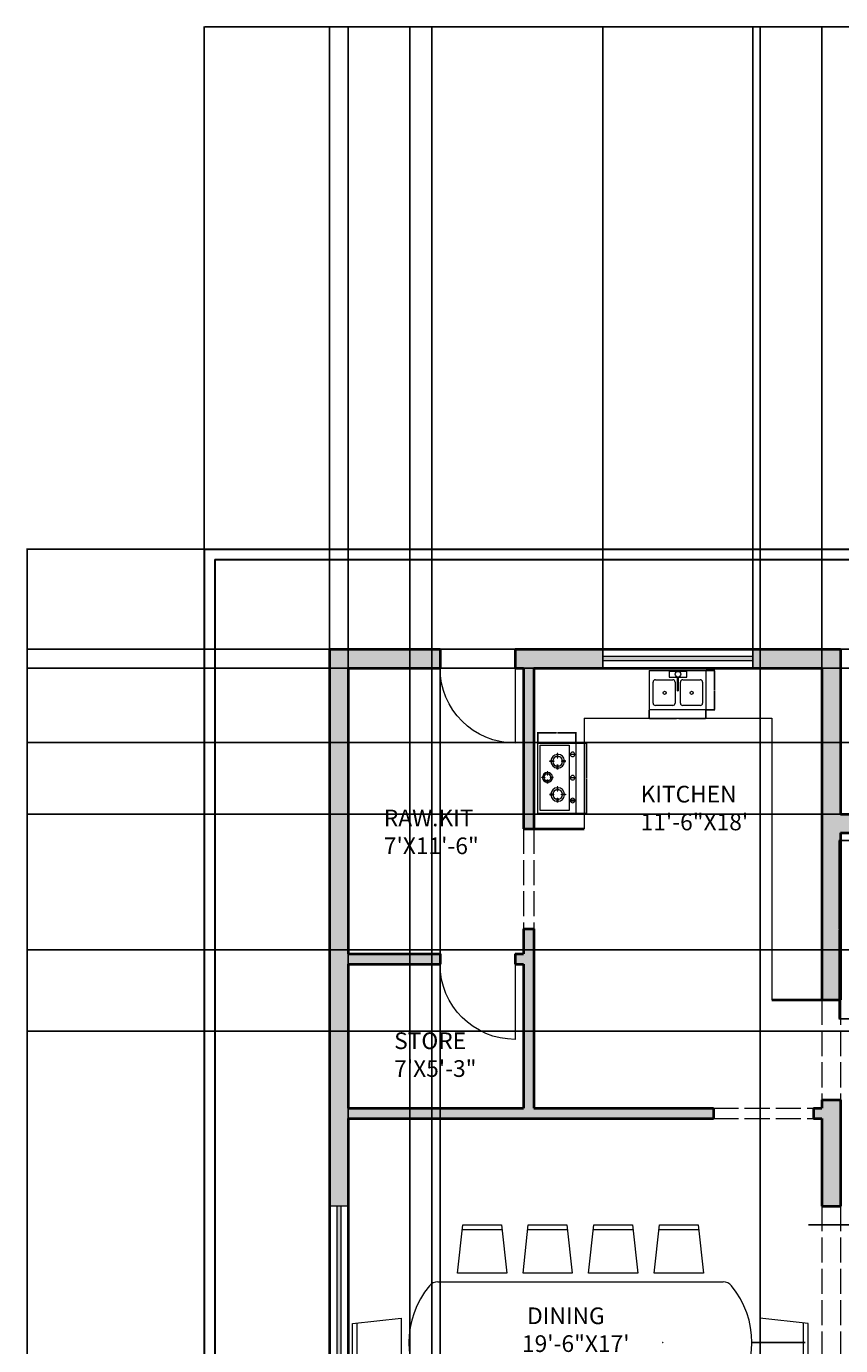
# Model space of a CAD drawing. Units: inches. Extents: x 2330 to 3943, y 1763 to 3461.
# Tile 24 of 40: x 2330 to 2721, y 2829 to 3461. Entities that reach past the tile are written whole.
import ezdxf

# ---------------------------------------------------------------- set-up
doc = ezdxf.new("R2010")
doc.units = ezdxf.units.IN
doc.linetypes.add('ACAD_ISO02W100', pattern=[15, 12, -3])
for name, color, linetype, lineweight in [('A-ANNO-DIMS', 2, 'Continuous', 18), ('A-AREA-IDEN', 7, 'Continuous', 18), ('A-DOOR', 4, 'Continuous', 18), ('A-EQPM', 9, 'Continuous', 18), ('A-FLOR-CASE', 8, 'Continuous', 18), ('A-FLOR-FIXT', 8, 'Continuous', 18), ('A-FURN', 8, 'Continuous', 13), ('A-GLAZ', 4, 'Continuous', 18), ('A-WALL', 7, 'Continuous', 40), ('A-WALL-OVHD', 7, 'ACAD_ISO02W100', 18), ('A-WALL-PATT', 252, 'Continuous', 13), ('C-PROP', 7, 'Continuous', 30)]:
    doc.layers.add(name, color=color, linetype=linetype, lineweight=lineweight)
doc.styles.get("Standard").update_dxf_attribs({"font": 'arial.ttf'})
doc.dimstyles.get("Standard").update_dxf_attribs({"dimtxt": 0.18, "dimasz": 0.18, "dimexe": 0.18, "dimexo": 0.0625, "dimgap": 0.09, "dimtad": 0, "dimtih": 1, "dimtoh": 1, "dimdec": 4, "dimzin": 0, "dimdsep": 46, "dimtxsty": 'Standard', "dimcen": 0.09, "dimadec": 0, "dimazin": 0, "dimtfac": 1, "dimtdec": 4, "dimtofl": 0, "dimtmove": 0, "dimatfit": 3, "dimfxl": 1, "dimtolj": 1, "dimtzin": 0, "dimarcsym": 0})

# ---------------------------------------------------------------- blocks, each defined once
blk = doc.blocks.new('A$C113D154D')
for p, q in [((0.96, 1.712), (1.008, 2.155)), ((1.003, 2.112), (1.367, 2.112)), ((1.008, 2.155), (1.362, 2.155)), ((1.362, 2.155), (1.41, 1.712)), ((1.56, 1.712), (1.608, 2.155)), ((1.603, 2.112), (1.967, 2.112)), ((1.608, 2.155), (1.962, 2.155)), ((1.962, 2.155), (2.01, 1.712)), ((2.16, 1.712), (2.208, 2.155)), ((2.203, 2.112), (2.567, 2.112)), ((2.208, 2.155), (2.562, 2.155)), ((2.562, 2.155), (2.61, 1.712)), ((2.76, 1.712), (2.808, 2.155)), ((2.803, 2.112), (3.167, 2.112)), ((2.808, 2.155), (3.162, 2.155)), ((3.162, 2.155), (3.21, 1.712)), ((1.41, 1.712), (0.96, 1.712)), ((2.01, 1.712), (1.56, 1.712)), ((2.61, 1.712), (2.16, 1.712)), ((3.21, 1.712), (2.76, 1.712)), ((0.78, 1.633), (3.39, 1.633)), ((0, 1.252), (0.443, 1.3)), ((0, 0.897), (0, 1.252)), ((0.043, 0.893), (0.043, 1.257)), ((0.443, 1.3), (0.443, 0.85)), ((3.727, 1.3), (3.727, 0.85)), ((4.17, 1.252), (3.727, 1.3)), ((4.127, 0.893), (4.127, 1.257)), ((4.17, 0.897), (4.17, 1.252)), ((0.443, 0.85), (0, 0.897)), ((3.727, 0.85), (4.17, 0.897)), ((3.39, 0.521), (0.78, 0.521)), ((1.41, 0.443), (0.96, 0.443)), ((0.96, 0.443), (1.008, 0)), ((1.362, 0), (1.41, 0.443)), ((2.01, 0.443), (1.56, 0.443)), ((1.56, 0.443), (1.608, 0)), ((1.962, 0), (2.01, 0.443)), ((2.61, 0.443), (2.16, 0.443)), ((2.16, 0.443), (2.208, 0)), ((2.562, 0), (2.61, 0.443)), ((3.21, 0.443), (2.76, 0.443)), ((2.76, 0.443), (2.808, 0)), ((3.162, 0), (3.21, 0.443)), ((1.003, 0.043), (1.367, 0.043)), ((1.008, 0), (1.362, 0)), ((1.603, 0.043), (1.967, 0.043)), ((1.608, 0), (1.962, 0)), ((2.203, 0.043), (2.567, 0.043)), ((2.208, 0), (2.562, 0)), ((2.803, 0.043), (3.167, 0.043)), ((2.808, 0), (3.162, 0))]:
    blk.add_line(p, q)
for centre, radius, start, end in [((1.331, 1.077), 0.815, 140.3976, 219.6024), ((0.78, 1.533), 0.1, 90, 140.3976), ((3.39, 1.533), 0.1, 39.6024, 90), ((2.839, 1.077), 0.815, 320.3976, 39.6024), ((0.78, 0.621), 0.1, 219.6024, 270), ((3.39, 0.621), 0.1, 270, 320.3976)]:
    blk.add_arc(centre, radius, start, end)
blk = doc.blocks.new('A$C72243D80')
at = {"ltscale": 1000}
for p, q in [((0, 0), (0, 384)), ((0, 384), (712, 384)), ((30, 69), (30, 363)), ((30, 363), (693, 363)), ((309, 291), (340, 291)), ((309, 285), (309, 291)), ((340, 285), (309, 285)), ((340, 291), (340, 285)), ((364, 315), (364, 345)), ((364, 345), (370, 345)), ((370, 315), (364, 315)), ((370, 345), (370, 315)), ((392, 291), (392, 285)), ((423, 291), (392, 291)), ((392, 285), (423, 285)), ((423, 285), (423, 291)), ((693, 363), (693, 69)), ((712, 384), (712, 0)), ((115, 190), (157, 190)), ((115, 182), (115, 190)), ((157, 182), (115, 182)), ((157, 190), (157, 182)), ((188, 264), (188, 222)), ((196, 264), (188, 264)), ((188, 222), (196, 222)), ((188, 147), (196, 147)), ((188, 105), (188, 147)), ((196, 222), (196, 264)), ((196, 147), (196, 105)), ((229, 190), (229, 182)), ((271, 190), (229, 190)), ((229, 182), (271, 182)), ((271, 182), (271, 190)), ((364, 260), (364, 229)), ((370, 260), (364, 260)), ((364, 229), (370, 229)), ((370, 229), (370, 260)), ((451, 190), (494, 190)), ((451, 182), (451, 190)), ((494, 182), (451, 182)), ((494, 190), (494, 182)), ((526, 222), (526, 264)), ((526, 264), (534, 264)), ((534, 222), (526, 222)), ((526, 147), (526, 105)), ((534, 147), (526, 147)), ((534, 264), (534, 222)), ((534, 105), (534, 147)), ((565, 190), (565, 182)), ((608, 190), (565, 190)), ((565, 182), (608, 182)), ((608, 182), (608, 190)), ((712, 0), (0, 0)), ((693, 69), (30, 69)), ((130, 61), (130, 5)), ((134, 61), (130, 61)), ((130, 5), (134, 5)), ((134, 5), (134, 61)), ((196, 105), (188, 105)), ((361, 5), (361, 61)), ((361, 61), (366, 61)), ((366, 5), (361, 5)), ((366, 61), (366, 5)), ((526, 105), (534, 105)), ((597, 5), (597, 61)), ((597, 61), (602, 61)), ((602, 5), (597, 5)), ((602, 61), (602, 5))]:
    blk.add_line(p, q, dxfattribs=at)
for centre, radius, start, end in [((366, 287), 50.3, 93.0344, 175.7271), ((366, 287), 50.3, 182.5783, 266.9656), ((366, 288), 36.3, 94.0374, 175.0142), ((366, 288), 36.3, 184.5153, 265.9626), ((366, 287), 50.3, 4.2729, 86.1838), ((366, 288), 36.3, 4.9858, 84.5356), ((366, 288), 36.3, 275.4644, 355.4847), ((366, 287), 50.3, 273.8162, 357.4217), ((193, 185), 69.2, 93.8162, 175.7271), ((193, 185), 69.2, 182.5783, 266.1838), ((193, 185), 49.9, 95.4644, 175.0142), ((193, 185), 49.9, 184.5153, 264.5356), ((193, 185), 69.2, 4.2729, 86.9656), ((193, 185), 49.9, 4.9858, 85.9626), ((193, 185), 49.9, 274.0374, 355.4847), ((193, 185), 69.2, 273.0344, 357.4217), ((530, 185), 69.2, 182.5783, 266.9656), ((530, 185), 69.2, 93.0344, 175.7271), ((529, 185), 49.9, 94.0374, 175.0142), ((529, 185), 49.9, 184.5153, 265.9626), ((530, 185), 69.2, 4.2729, 86.1838), ((529, 185), 49.9, 4.9858, 84.5356), ((530, 185), 69.2, 273.8162, 357.4217), ((529, 185), 49.9, 275.4644, 355.4847), ((132, 33), 22.5, 96.7453, 263.2547), ((132, 33), 22.5, 275.4789, 84.5211), ((363, 33), 22.5, 95.4789, 264.5211), ((363, 33), 22.5, 276.7453, 83.2547), ((599, 33), 22.5, 95.4789, 264.5211), ((599, 33), 22.5, 276.7453, 83.2547)]:
    blk.add_arc(centre, radius, start, end, dxfattribs=at)
blk = doc.blocks.new('A$C3AD04490')
for p, q in [((0, 641), (0, 0)), ((0, 641), (925, 641)), ((62, 111), (62, 451)), ((101, 490), (383, 490)), ((614, 627), (323, 627)), ((323, 627), (323, 532)), ((323, 532), (614, 532)), ((422, 451), (422, 111)), ((463, 312), (463, 537)), ((474, 537), (474, 312)), ((509, 111), (509, 451)), ((548, 490), (830, 490)), ((614, 532), (614, 627)), ((869, 451), (869, 111)), ((925, 641), (925, 0)), ((463, 311), (474, 311)), ((383, 72), (101, 72)), ((830, 72), (548, 72)), ((925, 0), (0, 0))]:
    blk.add_line(p, q)
for centre, radius in [((469, 581), 45.9), ((251, 278), 26.4), ((691, 278), 26.4)]:
    blk.add_circle(centre, radius)
for centre, start, end in [((101, 451), 90, 180), ((383, 451), 0, 90), ((548, 451), 90, 180), ((830, 451), 0, 90), ((101, 111), 180, 270), ((383, 111), 270, 0), ((548, 111), 180, 270), ((830, 111), 270, 0)]:
    blk.add_arc(centre, 39.1, start, end)
blk = doc.blocks.new('DOOR-SINGLE-36IN')
blk.add_line((0, 0), (-36, 0))
blk.add_arc((0, 0), 36, 180, 270)
blk = doc.blocks.new('WINDOW-120IN')
h = blk.add_hatch(color=256)
h.dxf.hatch_style = 1
h.paths.add_polyline_path([(120, 5.5), (0, 5.5), (0, 3.5), (120, 3.5)])
for p, q in [((0, 9), (0, 0)), ((120, 9), (120, 0)), ((120, 5.5), (0, 5.5)), ((120, 3.5), (0, 3.5))]:
    blk.add_line(p, q)
blk = doc.blocks.new('*D42')
at = {"layer": 'A-ANNO-DIMS', "color": 0, "lineweight": -2, "transparency": 16777216}
for p, q in [((2732.75, 3071.05), (2719.8, 3071.05)), ((2719.98, 3070.87), (2719.98, 3028.47)), ((2719.98, 2985.7), (2719.98, 3028.1)), ((2732.75, 2985.52), (2719.8, 2985.52))]:
    blk.add_line(p, q, dxfattribs=at)
at = {"layer": 'A-ANNO-DIMS', "color": 0, "transparency": 16777216}
for points in [[(2719.95, 3070.87), (2720.01, 3070.87), (2719.98, 3071.05)], [(2719.95, 2985.7), (2720.01, 2985.7), (2719.98, 2985.52)]]:
    blk.add_solid(points, dxfattribs=at)
at = {"layer": 'Defpoints', "color": 0, "transparency": 16777216}
for p in [(2719.98, 3071.05), (2732.81, 3071.05), (2732.81, 2985.52)]:
    blk.add_point(p, dxfattribs=at)
at = {"layer": 'A-ANNO-DIMS', "color": 0, "transparency": 16777216, "insert": (2719.98, 3028.29), "char_height": 0.18, "attachment_point": 5}
blk.add_mtext('\\A1;86 TYP.', dxfattribs=at)
blk = doc.blocks.new('*D52')
at = {"layer": 'A-ANNO-DIMS', "color": 0, "lineweight": -2, "transparency": 16777216}
for p, q in [((2705.22, 2886.72), (2738.1, 2886.72)), ((2737.92, 2886.54), (2737.92, 2830.48)), ((2737.92, 2774.05), (2737.92, 2830.11)), ((2705.22, 2773.87), (2738.1, 2773.87))]:
    blk.add_line(p, q, dxfattribs=at)
at = {"layer": 'A-ANNO-DIMS', "color": 0, "transparency": 16777216}
for points in [[(2737.89, 2886.54), (2737.95, 2886.54), (2737.92, 2886.72)], [(2737.89, 2774.05), (2737.95, 2774.05), (2737.92, 2773.87)]]:
    blk.add_solid(points, dxfattribs=at)
at = {"layer": 'Defpoints', "color": 0, "transparency": 16777216}
for p in [(2705.15, 2886.72), (2737.92, 2886.72), (2705.15, 2773.87)]:
    blk.add_point(p, dxfattribs=at)
at = {"layer": 'A-ANNO-DIMS', "color": 0, "transparency": 16777216, "insert": (2737.92, 2830.3), "char_height": 0.18, "attachment_point": 5}
blk.add_mtext('\\A1;113', dxfattribs=at)
blk = doc.blocks.new('*D53')
at = {"layer": 'A-ANNO-DIMS', "color": 0, "lineweight": -2, "transparency": 16777216}
for p, q in [((2593.83, 3117.63), (2599, 3117.63)), ((2598.82, 3117.45), (2598.82, 3100.96)), ((2598.82, 3084.1), (2598.82, 3100.59)), ((2593.83, 3083.92), (2599, 3083.92))]:
    blk.add_line(p, q, dxfattribs=at)
at = {"layer": 'A-ANNO-DIMS', "color": 0, "transparency": 16777216}
for points in [[(2598.79, 3117.45), (2598.85, 3117.45), (2598.82, 3117.63)], [(2598.79, 3084.1), (2598.85, 3084.1), (2598.82, 3083.92)]]:
    blk.add_solid(points, dxfattribs=at)
at = {"layer": 'Defpoints', "color": 0, "transparency": 16777216}
for p in [(2593.76, 3117.63), (2598.82, 3117.63), (2593.76, 3083.92)]:
    blk.add_point(p, dxfattribs=at)
at = {"layer": 'A-ANNO-DIMS', "color": 0, "transparency": 16777216, "insert": (2598.82, 3100.77), "char_height": 0.18, "attachment_point": 5}
blk.add_mtext('\\A1;HOB 34', dxfattribs=at)
blk = doc.blocks.new('*D54')
at = {"layer": 'A-ANNO-DIMS', "color": 0, "lineweight": -2, "transparency": 16777216}
for p, q in [((2575.57, 3117.69), (2575.57, 3122.87)), ((2575.75, 3122.69), (2584.46, 3122.69)), ((2593.58, 3122.69), (2584.88, 3122.69)), ((2593.76, 3117.69), (2593.76, 3122.87))]:
    blk.add_line(p, q, dxfattribs=at)
at = {"layer": 'A-ANNO-DIMS', "color": 0, "transparency": 16777216}
for points in [[(2575.75, 3122.72), (2575.75, 3122.66), (2575.57, 3122.69)], [(2593.58, 3122.72), (2593.58, 3122.66), (2593.76, 3122.69)]]:
    blk.add_solid(points, dxfattribs=at)
at = {"layer": 'Defpoints', "color": 0, "transparency": 16777216}
for p in [(2575.57, 3122.69), (2575.57, 3117.63), (2593.76, 3117.63)]:
    blk.add_point(p, dxfattribs=at)
at = {"layer": 'A-ANNO-DIMS', "color": 0, "transparency": 16777216, "insert": (2584.67, 3122.69), "char_height": 0.18, "attachment_point": 5}
blk.add_mtext('\\A1;18', dxfattribs=at)
blk = doc.blocks.new('*D55')
at = {"layer": 'A-ANNO-DIMS', "color": 0, "lineweight": -2, "transparency": 16777216}
for p, q in [((2628.92, 3133.56), (2628.92, 3129.36)), ((2656.13, 3133.56), (2656.13, 3129.36)), ((2629.1, 3129.54), (2641.98, 3129.54)), ((2655.95, 3129.54), (2643.07, 3129.54))]:
    blk.add_line(p, q, dxfattribs=at)
at = {"layer": 'A-ANNO-DIMS', "color": 0, "transparency": 16777216}
for points in [[(2629.1, 3129.57), (2629.1, 3129.51), (2628.92, 3129.54)], [(2655.95, 3129.57), (2655.95, 3129.51), (2656.13, 3129.54)]]:
    blk.add_solid(points, dxfattribs=at)
at = {"layer": 'Defpoints', "color": 0, "transparency": 16777216}
for p in [(2628.92, 3133.62), (2656.13, 3133.62), (2656.13, 3129.54)]:
    blk.add_point(p, dxfattribs=at)
at = {"layer": 'A-ANNO-DIMS', "color": 0, "transparency": 16777216, "insert": (2642.52, 3129.54), "char_height": 0.18, "attachment_point": 5}
blk.add_mtext('\\A1;SINK 27', dxfattribs=at)
blk = doc.blocks.new('*D56')
at = {"layer": 'A-ANNO-DIMS', "color": 0, "lineweight": -2, "transparency": 16777216}
for p, q in [((2656.19, 3152.47), (2660.39, 3152.47)), ((2660.21, 3152.29), (2660.21, 3143.23)), ((2660.21, 3133.8), (2660.21, 3142.87)), ((2656.19, 3133.62), (2660.39, 3133.62))]:
    blk.add_line(p, q, dxfattribs=at)
at = {"layer": 'A-ANNO-DIMS', "color": 0, "transparency": 16777216}
for points in [[(2660.18, 3152.29), (2660.24, 3152.29), (2660.21, 3152.47)], [(2660.18, 3133.8), (2660.24, 3133.8), (2660.21, 3133.62)]]:
    blk.add_solid(points, dxfattribs=at)
at = {"layer": 'Defpoints', "color": 0, "transparency": 16777216}
for p in [(2656.13, 3152.47), (2660.21, 3152.47), (2656.13, 3133.62)]:
    blk.add_point(p, dxfattribs=at)
at = {"layer": 'A-ANNO-DIMS', "color": 0, "transparency": 16777216, "insert": (2660.21, 3143.05), "char_height": 0.18, "attachment_point": 5}
blk.add_mtext('\\A1;19', dxfattribs=at)
blk = doc.blocks.new('*D59')
at = {"layer": 'A-ANNO-DIMS', "color": 0, "lineweight": -2, "transparency": 16777216}
for p, q in [((2415.66, 3210.71), (2415.66, 3461.3)), ((2415.84, 3461.12), (3111.31, 3461.12)), ((3807.48, 3461.12), (3112.01, 3461.12)), ((3807.66, 3210.71), (3807.66, 3461.3))]:
    blk.add_line(p, q, dxfattribs=at)
at = {"layer": 'A-ANNO-DIMS', "color": 0, "transparency": 16777216}
for points in [[(2415.84, 3461.15), (2415.84, 3461.09), (2415.66, 3461.12)], [(3807.48, 3461.15), (3807.48, 3461.09), (3807.66, 3461.12)]]:
    blk.add_solid(points, dxfattribs=at)
at = {"layer": 'Defpoints', "color": 0, "transparency": 16777216}
for p in [(3807.66, 3461.12), (2415.66, 3210.65), (3807.66, 3210.65)]:
    blk.add_point(p, dxfattribs=at)
at = {"layer": 'A-ANNO-DIMS', "color": 0, "transparency": 16777216, "insert": (3111.66, 3461.12), "char_height": 0.18, "attachment_point": 5}
blk.add_mtext('\\A1;1392', dxfattribs=at)
blk = doc.blocks.new('*D60')
at = {"layer": 'A-ANNO-DIMS', "color": 0, "lineweight": -2, "transparency": 16777216}
for p, q in [((2415.6, 3210.65), (2330.5, 3210.65)), ((2330.68, 3210.47), (2330.68, 2592.83)), ((2330.68, 1974.83), (2330.68, 2592.47)), ((2415.6, 1974.65), (2330.5, 1974.65))]:
    blk.add_line(p, q, dxfattribs=at)
at = {"layer": 'A-ANNO-DIMS', "color": 0, "transparency": 16777216}
for points in [[(2330.65, 3210.47), (2330.71, 3210.47), (2330.68, 3210.65)], [(2330.65, 1974.83), (2330.71, 1974.83), (2330.68, 1974.65)]]:
    blk.add_solid(points, dxfattribs=at)
at = {"layer": 'Defpoints', "color": 0, "transparency": 16777216}
for p in [(2330.68, 3210.65), (2415.66, 3210.65), (2415.66, 1974.65)]:
    blk.add_point(p, dxfattribs=at)
at = {"layer": 'A-ANNO-DIMS', "color": 0, "transparency": 16777216, "insert": (2330.68, 2592.65), "char_height": 0.18, "attachment_point": 5}
blk.add_mtext('\\A1;1236', dxfattribs=at)
blk = doc.blocks.new('*D61')
at = {"layer": 'A-ANNO-DIMS', "color": 0, "lineweight": -2, "transparency": 16777216}
for p, q in [((2475.66, 3162.71), (2475.66, 3461.3)), ((2475.84, 3461.12), (2965.37, 3461.12)), ((3455.48, 3461.12), (2965.95, 3461.12)), ((3455.66, 3162.71), (3455.66, 3461.3))]:
    blk.add_line(p, q, dxfattribs=at)
at = {"layer": 'A-ANNO-DIMS', "color": 0, "transparency": 16777216}
for points in [[(2475.84, 3461.15), (2475.84, 3461.09), (2475.66, 3461.12)], [(3455.48, 3461.15), (3455.48, 3461.09), (3455.66, 3461.12)]]:
    blk.add_solid(points, dxfattribs=at)
at = {"layer": 'Defpoints', "color": 0, "transparency": 16777216}
for p in [(3455.66, 3461.12), (2475.66, 3162.65), (3455.66, 3162.65)]:
    blk.add_point(p, dxfattribs=at)
at = {"layer": 'A-ANNO-DIMS', "color": 0, "transparency": 16777216, "insert": (2965.66, 3461.12), "char_height": 0.18, "attachment_point": 5}
blk.add_mtext('\\A1;980', dxfattribs=at)
blk = doc.blocks.new('*D62')
at = {"layer": 'A-ANNO-DIMS', "color": 0, "lineweight": -2, "transparency": 16777216}
for p, q in [((2475.6, 3162.65), (2330.5, 3162.65)), ((2330.68, 3162.47), (2330.68, 2687.58)), ((2330.68, 2212.33), (2330.68, 2687.22)), ((2475.6, 2212.15), (2330.5, 2212.15))]:
    blk.add_line(p, q, dxfattribs=at)
at = {"layer": 'A-ANNO-DIMS', "color": 0, "transparency": 16777216}
for points in [[(2330.65, 3162.47), (2330.71, 3162.47), (2330.68, 3162.65)], [(2330.65, 2212.33), (2330.71, 2212.33), (2330.68, 2212.15)]]:
    blk.add_solid(points, dxfattribs=at)
at = {"layer": 'Defpoints', "color": 0, "transparency": 16777216}
for p in [(2330.68, 3162.65), (2475.66, 3162.65), (2475.66, 2212.15)]:
    blk.add_point(p, dxfattribs=at)
at = {"layer": 'A-ANNO-DIMS', "color": 0, "transparency": 16777216, "insert": (2330.68, 2687.4), "char_height": 0.18, "attachment_point": 5}
blk.add_mtext('\\A1;950.5', dxfattribs=at)
blk = doc.blocks.new('*D63')
at = {"layer": 'A-ANNO-DIMS', "color": 0, "lineweight": -2, "transparency": 16777216}
for p, q in [((2415.66, 3210.71), (2415.66, 3461.3)), ((2415.84, 3461.12), (2445.44, 3461.12)), ((2475.48, 3461.12), (2445.88, 3461.12)), ((2475.66, 3162.71), (2475.66, 3461.3))]:
    blk.add_line(p, q, dxfattribs=at)
at = {"layer": 'A-ANNO-DIMS', "color": 0, "transparency": 16777216}
for points in [[(2415.84, 3461.15), (2415.84, 3461.09), (2415.66, 3461.12)], [(2475.48, 3461.15), (2475.48, 3461.09), (2475.66, 3461.12)]]:
    blk.add_solid(points, dxfattribs=at)
at = {"layer": 'Defpoints', "color": 0, "transparency": 16777216}
for p in [(2475.66, 3461.12), (2415.66, 3210.65), (2475.66, 3162.65)]:
    blk.add_point(p, dxfattribs=at)
at = {"layer": 'A-ANNO-DIMS', "color": 0, "transparency": 16777216, "insert": (2445.66, 3461.12), "char_height": 0.18, "attachment_point": 5}
blk.add_mtext('\\A1;60', dxfattribs=at)
blk = doc.blocks.new('*D64')
at = {"layer": 'A-ANNO-DIMS', "color": 0, "lineweight": -2, "transparency": 16777216}
for p, q in [((2415.6, 3210.65), (2330.5, 3210.65)), ((2330.68, 3210.47), (2330.68, 3186.83)), ((2330.68, 3162.83), (2330.68, 3186.47)), ((2475.6, 3162.65), (2330.5, 3162.65))]:
    blk.add_line(p, q, dxfattribs=at)
at = {"layer": 'A-ANNO-DIMS', "color": 0, "transparency": 16777216}
for points in [[(2330.65, 3210.47), (2330.71, 3210.47), (2330.68, 3210.65)], [(2330.65, 3162.83), (2330.71, 3162.83), (2330.68, 3162.65)]]:
    blk.add_solid(points, dxfattribs=at)
at = {"layer": 'Defpoints', "color": 0, "transparency": 16777216}
for p in [(2415.66, 3210.65), (2330.68, 3162.65), (2475.66, 3162.65)]:
    blk.add_point(p, dxfattribs=at)
at = {"layer": 'A-ANNO-DIMS', "color": 0, "transparency": 16777216, "insert": (2330.68, 3186.65), "char_height": 0.18, "attachment_point": 5}
blk.add_mtext('\\A1;48', dxfattribs=at)
blk = doc.blocks.new('*D76')
at = {"layer": 'A-ANNO-DIMS', "color": 0, "lineweight": -2, "transparency": 16777216}
for p, q in [((2968.6, 3162.65), (2330.5, 3162.65)), ((2330.68, 3162.47), (2330.68, 3123.33)), ((2330.68, 3083.83), (2330.68, 3122.97)), ((2968.6, 3083.65), (2330.5, 3083.65))]:
    blk.add_line(p, q, dxfattribs=at)
at = {"layer": 'A-ANNO-DIMS', "color": 0, "transparency": 16777216}
for points in [[(2330.65, 3162.47), (2330.71, 3162.47), (2330.68, 3162.65)], [(2330.65, 3083.83), (2330.71, 3083.83), (2330.68, 3083.65)]]:
    blk.add_solid(points, dxfattribs=at)
at = {"layer": 'Defpoints', "color": 0, "transparency": 16777216}
for p in [(2330.68, 3162.65), (2968.66, 3162.65), (2968.66, 3083.65)]:
    blk.add_point(p, dxfattribs=at)
at = {"layer": 'A-ANNO-DIMS', "color": 0, "transparency": 16777216, "insert": (2330.68, 3123.15), "char_height": 0.18, "attachment_point": 5}
blk.add_mtext('\\A1;79', dxfattribs=at)
blk = doc.blocks.new('*D79')
at = {"layer": 'A-ANNO-DIMS', "color": 0, "lineweight": -2, "transparency": 16777216}
for p, q in [((2484.66, 2221.21), (2484.66, 3461.3)), ((2484.84, 3461.12), (2504.44, 3461.12)), ((2524.48, 3461.12), (2504.88, 3461.12)), ((2524.66, 2221.21), (2524.66, 3461.3))]:
    blk.add_line(p, q, dxfattribs=at)
at = {"layer": 'A-ANNO-DIMS', "color": 0, "transparency": 16777216}
for points in [[(2484.84, 3461.15), (2484.84, 3461.09), (2484.66, 3461.12)], [(2524.48, 3461.15), (2524.48, 3461.09), (2524.66, 3461.12)]]:
    blk.add_solid(points, dxfattribs=at)
at = {"layer": 'Defpoints', "color": 0, "transparency": 16777216}
for p in [(2524.66, 3461.12), (2484.66, 2221.15), (2524.66, 2221.15)]:
    blk.add_point(p, dxfattribs=at)
at = {"layer": 'A-ANNO-DIMS', "color": 0, "transparency": 16777216, "insert": (2504.66, 3461.12), "char_height": 0.18, "attachment_point": 5}
blk.add_mtext('\\A1;40', dxfattribs=at)
blk = doc.blocks.new('*D83')
at = {"layer": 'A-ANNO-DIMS', "color": 0, "lineweight": -2, "transparency": 16777216}
for p, q in [((2514.16, 2733.71), (2514.16, 3461.3)), ((2514.34, 3461.12), (2597.88, 3461.12)), ((2681.98, 3461.12), (2598.44, 3461.12)), ((2682.16, 2733.71), (2682.16, 3461.3))]:
    blk.add_line(p, q, dxfattribs=at)
at = {"layer": 'A-ANNO-DIMS', "color": 0, "transparency": 16777216}
for points in [[(2514.34, 3461.15), (2514.34, 3461.09), (2514.16, 3461.12)], [(2681.98, 3461.15), (2681.98, 3461.09), (2682.16, 3461.12)]]:
    blk.add_solid(points, dxfattribs=at)
at = {"layer": 'Defpoints', "color": 0, "transparency": 16777216}
for p in [(2682.16, 3461.12), (2514.16, 2733.65), (2682.16, 2733.65)]:
    blk.add_point(p, dxfattribs=at)
at = {"layer": 'A-ANNO-DIMS', "color": 0, "transparency": 16777216, "insert": (2598.16, 3461.12), "char_height": 0.18, "attachment_point": 5}
blk.add_mtext('\\A1;168', dxfattribs=at)
blk = doc.blocks.new('*D84')
at = {"layer": 'A-ANNO-DIMS', "color": 0, "lineweight": -2, "transparency": 16777216}
for p, q in [((2484.66, 2733.71), (2484.66, 3461.3)), ((2484.84, 3461.12), (2499.08, 3461.12)), ((2513.98, 3461.12), (2499.74, 3461.12)), ((2514.16, 2733.71), (2514.16, 3461.3))]:
    blk.add_line(p, q, dxfattribs=at)
at = {"layer": 'A-ANNO-DIMS', "color": 0, "transparency": 16777216}
for points in [[(2484.84, 3461.15), (2484.84, 3461.09), (2484.66, 3461.12)], [(2513.98, 3461.15), (2513.98, 3461.09), (2514.16, 3461.12)]]:
    blk.add_solid(points, dxfattribs=at)
at = {"layer": 'Defpoints', "color": 0, "transparency": 16777216}
for p in [(2514.16, 3461.12), (2484.66, 2733.65), (2514.16, 2733.65)]:
    blk.add_point(p, dxfattribs=at)
at = {"layer": 'A-ANNO-DIMS', "color": 0, "transparency": 16777216, "insert": (2499.41, 3461.12), "char_height": 0.18, "attachment_point": 5}
blk.add_mtext('\\A1;29.5', dxfattribs=at)
blk = doc.blocks.new('*D85')
at = {"layer": 'A-ANNO-DIMS', "color": 0, "lineweight": -2, "transparency": 16777216}
for p, q in [((3091.6, 3153.65), (2330.5, 3153.65)), ((2330.68, 3153.47), (2330.68, 3136.04)), ((2330.68, 3118.24), (2330.68, 3135.67)), ((3091.6, 3118.06), (2330.5, 3118.06))]:
    blk.add_line(p, q, dxfattribs=at)
at = {"layer": 'A-ANNO-DIMS', "color": 0, "transparency": 16777216}
for points in [[(2330.65, 3153.47), (2330.71, 3153.47), (2330.68, 3153.65)], [(2330.65, 3118.24), (2330.71, 3118.24), (2330.68, 3118.06)]]:
    blk.add_solid(points, dxfattribs=at)
at = {"layer": 'Defpoints', "color": 0, "transparency": 16777216}
for p in [(2330.68, 3153.65), (3091.66, 3153.65), (3091.66, 3118.06)]:
    blk.add_point(p, dxfattribs=at)
at = {"layer": 'A-ANNO-DIMS', "color": 0, "transparency": 16777216, "insert": (2330.68, 3135.86), "char_height": 0.18, "attachment_point": 5}
blk.add_mtext('\\A1;35.59', dxfattribs=at)
blk = doc.blocks.new('*D88')
at = {"layer": 'A-ANNO-DIMS', "color": 0, "lineweight": -2, "transparency": 16777216}
for p, q in [((2606.66, 3153.71), (2606.66, 3461.3)), ((2606.84, 3461.12), (2642.44, 3461.12)), ((2678.48, 3461.12), (2642.88, 3461.12)), ((2678.66, 3153.71), (2678.66, 3461.3))]:
    blk.add_line(p, q, dxfattribs=at)
at = {"layer": 'A-ANNO-DIMS', "color": 0, "transparency": 16777216}
for points in [[(2606.84, 3461.15), (2606.84, 3461.09), (2606.66, 3461.12)], [(2678.48, 3461.15), (2678.48, 3461.09), (2678.66, 3461.12)]]:
    blk.add_solid(points, dxfattribs=at)
at = {"layer": 'Defpoints', "color": 0, "transparency": 16777216}
for p in [(2678.66, 3461.12), (2606.66, 3153.65), (2678.66, 3153.65)]:
    blk.add_point(p, dxfattribs=at)
at = {"layer": 'A-ANNO-DIMS', "color": 0, "transparency": 16777216, "insert": (2642.66, 3461.12), "char_height": 0.18, "attachment_point": 5}
blk.add_mtext('\\A1;72', dxfattribs=at)
blk = doc.blocks.new('*D89')
at = {"layer": 'A-ANNO-DIMS', "color": 0, "lineweight": -2, "transparency": 16777216}
for p, q in [((2678.66, 3153.71), (2678.66, 3461.3)), ((2678.84, 3461.12), (2694.94, 3461.12)), ((2711.48, 3461.12), (2695.38, 3461.12)), ((2711.66, 3153.71), (2711.66, 3461.3))]:
    blk.add_line(p, q, dxfattribs=at)
at = {"layer": 'A-ANNO-DIMS', "color": 0, "transparency": 16777216}
for points in [[(2678.84, 3461.15), (2678.84, 3461.09), (2678.66, 3461.12)], [(2711.48, 3461.15), (2711.48, 3461.09), (2711.66, 3461.12)]]:
    blk.add_solid(points, dxfattribs=at)
at = {"layer": 'Defpoints', "color": 0, "transparency": 16777216}
for p in [(2711.66, 3461.12), (2678.66, 3153.65), (2711.66, 3153.65)]:
    blk.add_point(p, dxfattribs=at)
at = {"layer": 'A-ANNO-DIMS', "color": 0, "transparency": 16777216, "insert": (2695.16, 3461.12), "char_height": 0.18, "attachment_point": 5}
blk.add_mtext('\\A1;33', dxfattribs=at)
blk = doc.blocks.new('*D90')
at = {"layer": 'A-ANNO-DIMS', "color": 0, "lineweight": -2, "transparency": 16777216}
for p, q in [((2484.66, 3153.59), (2484.66, 1901.2)), ((2528.66, 3153.59), (2528.66, 1901.2)), ((2484.84, 1901.38), (2506.44, 1901.38)), ((2528.48, 1901.38), (2506.88, 1901.38))]:
    blk.add_line(p, q, dxfattribs=at)
at = {"layer": 'A-ANNO-DIMS', "color": 0, "transparency": 16777216}
for points in [[(2484.84, 1901.41), (2484.84, 1901.35), (2484.66, 1901.38)], [(2528.48, 1901.41), (2528.48, 1901.35), (2528.66, 1901.38)]]:
    blk.add_solid(points, dxfattribs=at)
at = {"layer": 'Defpoints', "color": 0, "transparency": 16777216}
for p in [(2484.66, 3153.65), (2528.66, 3153.65), (2528.66, 1901.38)]:
    blk.add_point(p, dxfattribs=at)
at = {"layer": 'A-ANNO-DIMS', "color": 0, "transparency": 16777216, "insert": (2506.66, 1901.38), "char_height": 0.18, "attachment_point": 5}
blk.add_mtext('\\A1;44', dxfattribs=at)
blk = doc.blocks.new('*D93')
at = {"layer": 'A-ANNO-DIMS', "color": 0, "lineweight": -2, "transparency": 16777216}
for p, q in [((3446.6, 3018.65), (2330.5, 3018.65)), ((2330.68, 3018.47), (2330.68, 2999.33)), ((2330.68, 2979.83), (2330.68, 2998.97)), ((3446.6, 2979.65), (2330.5, 2979.65))]:
    blk.add_line(p, q, dxfattribs=at)
at = {"layer": 'A-ANNO-DIMS', "color": 0, "transparency": 16777216}
for points in [[(2330.65, 3018.47), (2330.71, 3018.47), (2330.68, 3018.65)], [(2330.65, 2979.83), (2330.71, 2979.83), (2330.68, 2979.65)]]:
    blk.add_solid(points, dxfattribs=at)
at = {"layer": 'Defpoints', "color": 0, "transparency": 16777216}
for p in [(2330.68, 3018.65), (3446.66, 3018.65), (3446.66, 2979.65)]:
    blk.add_point(p, dxfattribs=at)
at = {"layer": 'A-ANNO-DIMS', "color": 0, "transparency": 16777216, "insert": (2330.68, 2999.15), "char_height": 0.18, "attachment_point": 5}
blk.add_mtext('\\A1;39', dxfattribs=at)
blk = doc.blocks.new('*D107')
at = {"layer": 'A-ANNO-DIMS', "color": 0, "lineweight": -2, "transparency": 16777216}
for p, q in [((2635.34, 2830.3), (2635.52, 2830.3)), ((2635.43, 2830.21), (2635.43, 2830.39)), ((2703.74, 2830.29), (2678.31, 2830.29))]:
    blk.add_line(p, q, dxfattribs=at)
at = {"layer": 'A-ANNO-DIMS', "color": 0, "transparency": 16777216}
blk.add_solid([(2678.31, 2830.32), (2678.31, 2830.26), (2678.13, 2830.29)], dxfattribs=at)
at = {"layer": 'Defpoints', "color": 0, "transparency": 16777216}
for p in [(2635.43, 2830.3), (2678.13, 2830.29)]:
    blk.add_point(p, dxfattribs=at)
at = {"layer": 'A-ANNO-DIMS', "color": 0, "transparency": 16777216, "insert": (2704.35, 2830.29), "char_height": 0.18, "attachment_point": 5}
blk.add_mtext('\\A1;2X R42.7', dxfattribs=at)

msp = doc.modelspace()

# ---------------------------------------------------------------- hatches: boundary and pattern name
at = {"layer": 'A-GLAZ'}
h = msp.add_hatch(color=256, dxfattribs=at)
h.dxf.hatch_style = 1
h.paths.add_polyline_path([(2678.6605, 3159.1524), (2606.6605, 3159.1524), (2606.6605, 3157.1524), (2678.6605, 3157.1524)])
at = {"layer": 'A-WALL-PATT'}
h = msp.add_hatch(color=256, dxfattribs=at)
h.dxf.hatch_style = 1
h.paths.add_polyline_path([(2573.6605, 3028.6524), (2568.6605, 3028.6524), (2568.6605, 3016.6524), (2564.6605, 3016.6524), (2564.6605, 3011.6524), (2568.6605, 3011.6524), (2568.6605, 2942.6524), (2484.6605, 2942.6524), (2484.6605, 3011.6524), (2528.6605, 3011.6524), (2528.6605, 3016.6524), (2484.6605, 3016.6524), (2484.6605, 3153.6524), (2528.6605, 3153.6524), (2528.6605, 3162.6524), (2475.6605, 3162.6524), (2475.6605, 2895.6524), (2484.6605, 2895.6524), (2484.6605, 2937.6524), (2659.6605, 2937.6524), (2659.6605, 2942.6524), (2573.6605, 2942.6524)])
h = msp.add_hatch(color=256, dxfattribs=at)
h.dxf.hatch_style = 1
h.paths.add_polyline_path([(2606.6605, 3162.6524), (2564.6605, 3162.6524), (2564.6605, 3153.6524), (2568.6605, 3153.6524), (2568.6605, 3076.6524), (2573.6605, 3076.6524), (2573.6605, 3153.6524), (2606.6605, 3153.6524)])
h = msp.add_hatch(color=256, dxfattribs=at)
h.dxf.hatch_style = 1
h.paths.add_polyline_path([(2772.6605, 3083.6524), (2720.6605, 3083.6524), (2720.6605, 3162.6524), (2678.6605, 3162.6524), (2678.6605, 3153.6524), (2711.6605, 3153.6524), (2711.6605, 2994.6524), (2720.6605, 2994.6524), (2720.6605, 3074.6524), (2772.6605, 3074.6524)])
h = msp.add_hatch(color=256, dxfattribs=at)
h.dxf.hatch_style = 1
h.paths.add_polyline_path([(2720.6605, 2946.6524), (2711.6605, 2946.6524), (2711.6605, 2942.6524), (2707.6605, 2942.6524), (2707.6605, 2937.6524), (2711.6605, 2937.6524), (2711.6605, 2895.6524), (2720.6605, 2895.6524)])

# ---------------------------------------------------------------- linework, layer by layer
at = {"layer": 'A-FLOR-CASE'}
for p, q in [((2597.6605, 3129.6524), (2687.6605, 3129.6524)), ((2597.6605, 3129.6524), (2597.6605, 3076.6524)), ((2687.6605, 3129.6524), (2687.6605, 2994.6524))]:
    msp.add_line(p, q, dxfattribs=at)
at = {"layer": 'A-GLAZ'}
for p, q in [((2606.6605, 3153.6524), (2606.6605, 3162.6524)), ((2678.6605, 3153.6524), (2678.6605, 3162.6524)), ((2678.6605, 3159.1524), (2606.6605, 3159.1524)), ((2678.6605, 3157.1524), (2606.6605, 3157.1524))]:
    msp.add_line(p, q, dxfattribs=at)
at = {"layer": 'A-WALL'}
for p, q in [((2475.6605, 3162.6524), (2475.6605, 2212.1524)), ((2475.6605, 3162.6524), (2528.6605, 3162.6524)), ((2528.6605, 3162.6524), (2528.6605, 3153.6524)), ((2564.6605, 3162.6524), (2564.6605, 3153.6524)), ((2564.6605, 3162.6524), (2720.6605, 3162.6524)), ((2720.6605, 3162.6524), (2720.6605, 3083.6524)), ((2484.6605, 3153.6524), (2484.6605, 3016.6524)), ((2484.6605, 3153.6524), (2528.6605, 3153.6524)), ((2564.6605, 3153.6524), (2568.6605, 3153.6524)), ((2568.6605, 3153.6524), (2568.6605, 3076.6524)), ((2573.6605, 3153.6524), (2573.6605, 3076.6524)), ((2573.6605, 3153.6524), (2711.6605, 3153.6524)), ((2711.6605, 3153.6524), (2711.6605, 2994.6524)), ((2720.6605, 3083.6524), (2968.6605, 3083.6524)), ((2568.6605, 3076.6524), (2597.6605, 3076.6524)), ((2720.6605, 3074.6524), (2968.6605, 3074.6524)), ((2720.6605, 3074.6524), (2720.6605, 2994.6524)), ((2568.6605, 3028.6524), (2573.6605, 3028.6524)), ((2568.6605, 3028.6524), (2568.6605, 3016.6524)), ((2573.6605, 3028.6524), (2573.6605, 2942.6524)), ((2484.6605, 3016.6524), (2528.6605, 3016.6524)), ((2484.6605, 3011.6524), (2528.6605, 3011.6524)), ((2484.6605, 3011.6524), (2484.6605, 2942.6524)), ((2528.6605, 3016.6524), (2528.6605, 3011.6524)), ((2564.6605, 3016.6524), (2564.6605, 3011.6524)), ((2564.6605, 3016.6524), (2568.6605, 3016.6524)), ((2564.6605, 3011.6524), (2568.6605, 3011.6524)), ((2568.6605, 3011.6524), (2568.6605, 2942.6524)), ((2687.6605, 2994.6524), (2720.6605, 2994.6524)), ((2484.6605, 2942.6524), (2568.6605, 2942.6524)), ((2573.6605, 2942.6524), (2659.6605, 2942.6524)), ((2659.6605, 2942.6524), (2659.6605, 2937.6524)), ((2707.6605, 2942.6524), (2707.6605, 2937.6524)), ((2707.6605, 2942.6524), (2711.6605, 2942.6524)), ((2711.6605, 2946.6524), (2720.6605, 2946.6524)), ((2711.6605, 2946.6524), (2711.6605, 2942.6524)), ((2720.6605, 2946.6524), (2720.6605, 2895.6524)), ((2484.6605, 2937.6524), (2659.6605, 2937.6524)), ((2484.6605, 2937.6524), (2484.6605, 2733.6524)), ((2707.6605, 2937.6524), (2711.6605, 2937.6524)), ((2711.6605, 2937.6524), (2711.6605, 2895.6524)), ((2711.6605, 2895.6524), (2720.6605, 2895.6524))]:
    msp.add_line(p, q, dxfattribs=at)
at = {"layer": 'A-WALL-OVHD'}
for p, q in [((2568.6605, 3076.6524), (2568.6605, 3028.6524)), ((2573.6605, 3076.6524), (2573.6605, 3028.6524)), ((2711.6605, 2994.6524), (2711.6605, 2946.6524)), ((2720.6605, 2994.6524), (2720.6605, 2946.6524)), ((2659.6605, 2942.6524), (2707.6605, 2942.6524)), ((2659.6605, 2937.6524), (2707.6605, 2937.6524)), ((2711.6605, 2895.6524), (2711.6605, 2775.6524)), ((2720.6605, 2895.6524), (2720.6605, 2775.6524))]:
    msp.add_line(p, q, dxfattribs=at)
at = {"layer": 'C-PROP'}
for p, q in [((2415.6605, 3210.6524), (3807.6605, 3210.6524)), ((2415.6605, 3210.6524), (2415.6605, 1974.6524)), ((2420.6605, 3205.6524), (2420.6605, 1979.6524)), ((2420.6605, 3205.6524), (3802.6605, 3205.6524))]:
    msp.add_line(p, q, dxfattribs=at)

# ---------------------------------------------------------------- block references
at = {"layer": 'A-DOOR', "extrusion": (0, 0, -1), "zscale": -1, "rotation": 90.00000000000074}
for p in [(-2564.6605, 3153.6524), (-2564.6605, 3011.6524)]:
    msp.add_blockref('DOOR-SINGLE-36IN', p, dxfattribs=at)
at = {"layer": 'A-EQPM', "xscale": 0.0473494785343784, "yscale": 0.0473494785343784, "zscale": 0.0473494785343784, "rotation": 90}
msp.add_blockref('A$C72243D80', (2593.7633, 3083.916), dxfattribs=at)
at = {"layer": 'A-FLOR-FIXT', "xscale": 0.0294194925705446, "yscale": 0.0294194925705446, "zscale": 0.0294194925705446}
msp.add_blockref('A$C3AD04490', (2628.9188, 3133.6239), dxfattribs=at)
at = {"layer": 'A-FURN', "xscale": 52.37726238140837, "yscale": 52.37726238140837, "zscale": 52.37726238140837}
msp.add_blockref('A$C113D154D', (2486.7408, 2773.8664), dxfattribs=at)
at = {"layer": 'A-GLAZ', "extrusion": (0, 0, -1), "zscale": -1, "rotation": 90.00000000000006}
msp.add_blockref('WINDOW-120IN', (-2475.6605, 2775.6524), dxfattribs=at)

# ---------------------------------------------------------------- texts
at = {"layer": 'A-AREA-IDEN', "char_height": 8, "attachment_point": 1}
for s, width, insert in [('KITCHEN\\P11\'-6"X18\'', 95.863439, (2624.797, 3097.2287)), ('RAW.KIT\\P7\'X11\'-6"', 52.023455, (2501.7066, 3085.7924)), ('STORE\\P7\'X5\'-3"', 70.677681, (2506.6634, 2979.0011)), (' DINING\\P19\'-6"X17\'', 93.76933, (2567.9313, 2847.1316))]:
    msp.add_mtext_dynamic_manual_height_columns(s, width=width, gutter_width=12.5, heights=[0], dxfattribs=dict(at, insert=insert))

# ---------------------------------------------------------------- dimensions: what is measured, and where the dimension line sits
at = {"layer": 'A-ANNO-DIMS'}
for base, p1, p2, override, picture, middle in [((3807.6605, 3461.1231), (2415.6605, 3210.6524), (3807.6605, 3210.6524), {"dimdec": 0, "dimlfac": 1, "dimrnd": 0, "dimzin": 0, "dimdsep": 46, "dimlunit": 2}, '*D59', (3111.6605, 3461.1231)), ((2475.6605, 3461.1231), (2415.6605, 3210.6524), (2475.6605, 3162.6524), {"dimdec": 0, "dimlfac": 1, "dimrnd": 0, "dimzin": 0, "dimdsep": 46, "dimlunit": 2}, '*D63', (2445.6605, 3461.1231)), ((3455.6605, 3461.1231), (2475.6605, 3162.6524), (3455.6605, 3162.6524), {"dimdec": 0, "dimlfac": 1, "dimrnd": 0, "dimzin": 0, "dimdsep": 46, "dimlunit": 2}, '*D61', (2965.6605, 3461.1231)), ((2524.6605, 3461.1231), (2484.6605, 2221.1524), (2524.6605, 2221.1524), {"dimdec": 0, "dimlfac": 1, "dimrnd": 0, "dimzin": 0, "dimdsep": 46, "dimlunit": 2}, '*D79', (2504.6605, 3461.1231)), ((2514.1605, 3461.1231), (2484.6605, 2733.6524), (2514.1605, 2733.6524), {"dimdec": 1, "dimlfac": 1, "dimrnd": 0, "dimzin": 0, "dimdsep": 46, "dimlunit": 2}, '*D84', (2499.4105, 3461.1231)), ((2682.1605, 3461.1231), (2514.1605, 2733.6524), (2682.1605, 2733.6524), {"dimdec": 0, "dimlfac": 1, "dimrnd": 0, "dimzin": 0, "dimdsep": 46, "dimlunit": 2}, '*D83', (2598.1605, 3461.1231)), ((2678.6605, 3461.1231), (2606.6605, 3153.6524), (2678.6605, 3153.6524), {"dimdec": 0, "dimlfac": 1, "dimrnd": 0, "dimzin": 0, "dimdsep": 46, "dimlunit": 2}, '*D88', (2642.6605, 3461.1231)), ((2711.6605, 3461.1231), (2678.6605, 3153.6524), (2711.6605, 3153.6524), {"dimdec": 0, "dimlfac": 1, "dimrnd": 0, "dimzin": 0, "dimdsep": 46, "dimlunit": 2}, '*D89', (2695.1605, 3461.1231)), ((2528.6605, 1901.3774), (2484.6605, 3153.6524), (2528.6605, 3153.6524), {"dimdec": 0, "dimlfac": 1, "dimrnd": 0, "dimzin": 0, "dimdsep": 46, "dimlunit": 2}, '*D90', (2506.6605, 1901.3774))]:
    dim = msp.add_linear_dim(base=base, p1=p1, p2=p2, dimstyle='Standard', override=override, dxfattribs=at)
    dim.commit()
    dim.dimension.update_dxf_attribs({"geometry": picture, "text_midpoint": middle})
for base, p1, p2, angle, override, picture, middle in [((2330.6824, 3210.6524), (2415.6605, 1974.6524), (2415.6605, 3210.6524), 90, {"dimdec": 0, "dimlfac": 1, "dimrnd": 0, "dimzin": 0, "dimdsep": 46, "dimlunit": 2}, '*D60', (2330.6824, 2592.6524)), ((2330.6824, 3162.6524), (2415.6605, 3210.6524), (2475.6605, 3162.6524), 90, {"dimdec": 0, "dimlfac": 1, "dimrnd": 0, "dimzin": 0, "dimdsep": 46, "dimlunit": 2}, '*D64', (2330.6824, 3186.6524)), ((2330.6824, 3162.6524), (2475.6605, 2212.1524), (2475.6605, 3162.6524), 90, {"dimdec": 1, "dimlfac": 1, "dimrnd": 0, "dimzin": 0, "dimdsep": 46, "dimlunit": 2}, '*D62', (2330.6824, 2687.4024)), ((2330.6824, 3162.6524), (2968.6605, 3083.6524), (2968.6605, 3162.6524), 90, {"dimdec": 0, "dimlfac": 1, "dimrnd": 0, "dimzin": 0, "dimdsep": 46, "dimlunit": 2}, '*D76', (2330.6824, 3123.1524)), ((2330.6824, 3153.6524), (3091.6605, 3118.0598), (3091.6605, 3153.6524), 90, {"dimdec": 2, "dimlfac": 1, "dimrnd": 0, "dimzin": 0, "dimdsep": 46, "dimlunit": 2}, '*D85', (2330.6824, 3135.8561)), ((2660.2109, 3152.474), (2656.1294, 3133.6239), (2656.1294, 3152.474), 90, {"dimdec": 0, "dimlfac": 1, "dimrnd": 0, "dimzin": 0, "dimdsep": 46, "dimlunit": 2}, '*D56', (2660.2109, 3143.049)), ((2575.5713, 3122.6883), (2593.7633, 3117.631), (2575.5713, 3117.631), 180, {"dimdec": 0, "dimlfac": 1, "dimrnd": 0, "dimzin": 0, "dimdsep": 46, "dimlunit": 2}, '*D54', (2584.6673, 3122.6883)), ((2330.6824, 3018.6524), (3446.6605, 2979.6524), (3446.6605, 3018.6524), 90, {"dimdec": 0, "dimlfac": 1, "dimrnd": 0, "dimzin": 0, "dimdsep": 46, "dimlunit": 2}, '*D93', (2330.6824, 2999.1524)), ((2737.9166, 2886.7243), (2705.1545, 2773.8664), (2705.1545, 2886.7243), 90, {"dimdec": 0, "dimlfac": 1, "dimrnd": 0, "dimzin": 0, "dimdsep": 46, "dimlunit": 2}, '*D52', (2737.9166, 2830.2954))]:
    dim = msp.add_linear_dim(base=base, p1=p1, p2=p2, angle=angle, dimstyle='Standard', override=override, dxfattribs=at)
    dim.commit()
    dim.dimension.update_dxf_attribs({"geometry": picture, "text_midpoint": middle})
dim = msp.add_linear_dim(base=(2656.1294, 3129.5423), p1=(2628.9188, 3133.6239), p2=(2656.1294, 3133.6239), text='SINK <>', dimstyle='Standard', override={"dimdec": 0, "dimlfac": 1, "dimrnd": 0, "dimzin": 0, "dimdsep": 46, "dimlunit": 2}, dxfattribs=at)
dim.commit()
dim.dimension.update_dxf_attribs({"geometry": '*D55', "text_midpoint": (2642.5241, 3129.5423)})
for base, p1, p2, text, picture, middle in [((2598.8205, 3117.631), (2593.7633, 3083.916), (2593.7633, 3117.631), 'HOB <>', '*D53', (2598.8205, 3100.7735)), ((2719.9791, 3071.053), (2732.8094, 2985.5175), (2732.8094, 3071.053), '<> TYP.', '*D42', (2719.9791, 3028.2852))]:
    dim = msp.add_linear_dim(base=base, p1=p1, p2=p2, angle=90, text=text, dimstyle='Standard', override={"dimdec": 0, "dimlfac": 1, "dimrnd": 0, "dimzin": 0, "dimdsep": 46, "dimlunit": 2}, dxfattribs=at)
    dim.commit()
    dim.dimension.update_dxf_attribs({"geometry": picture, "text_midpoint": middle})
dim = msp.add_radius_dim(center=(2635.426, 2830.2954), mpoint=(2678.1252, 2830.295), text='2X <>', dimstyle='Standard', override={"dimdec": 1, "dimlfac": 1, "dimrnd": 0, "dimzin": 0, "dimdsep": 46, "dimlunit": 2}, dxfattribs=at)
dim.commit()
dim.dimension.update_dxf_attribs({"geometry": '*D107', "text_midpoint": (2703.7447, 2830.2948), "dimtype": 164})

doc.saveas('drawing.dxf')
